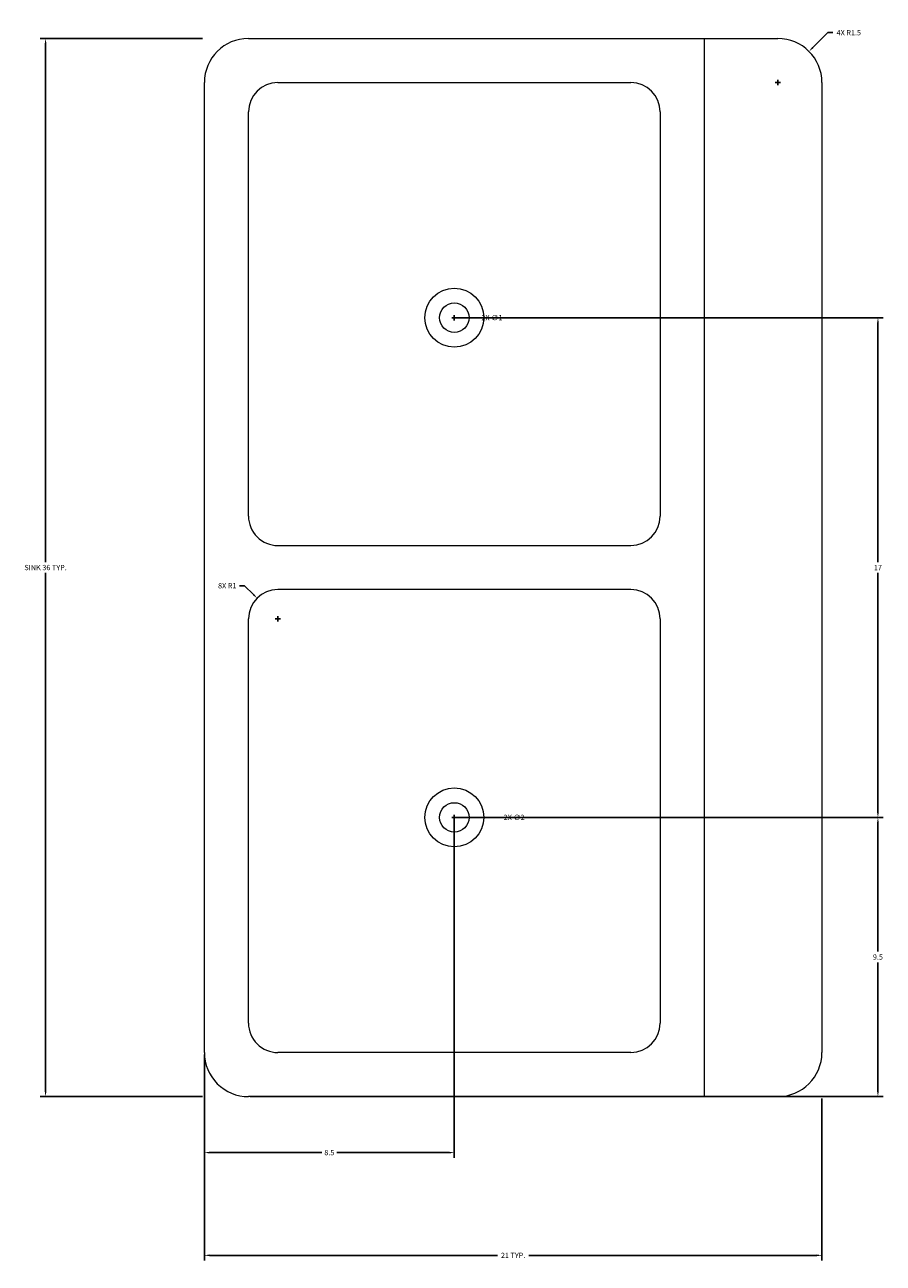
# Model space of a CAD drawing. Units: inches. Extents: x -494 to 1275, y 12 to 1194.
# Tile 8 of 8: x 1246 to 1275, y 824 to 866. Entities that reach past the tile are written whole.
import ezdxf

# ---------------------------------------------------------------- set-up
doc = ezdxf.new("R2010")
doc.units = ezdxf.units.IN
doc.header["$MEASUREMENT"] = 0
doc.layers.add('A-ANNO-DIMS', color=2, linetype='Continuous', lineweight=18)
doc.layers.add('A-FLOR-FIXT', color=8, linetype='Continuous', lineweight=18)
doc.styles.get("Standard").update_dxf_attribs({"font": 'arial.ttf'})
doc.dimstyles.get("Standard").update_dxf_attribs({"dimtxt": 0.18, "dimasz": 0.18, "dimexe": 0.18, "dimexo": 0.0625, "dimgap": 0.09, "dimtad": 0, "dimtih": 1, "dimtoh": 1, "dimdec": 4, "dimzin": 0, "dimdsep": 46, "dimlunit": 4, "dimtxsty": 'Standard', "dimcen": 0.09, "dimadec": 0, "dimazin": 0, "dimtfac": 1, "dimtdec": 4, "dimtofl": 0, "dimtmove": 0, "dimatfit": 3, "dimfxl": 1, "dimtolj": 1, "dimtzin": 0, "dimarcsym": 0})

# ---------------------------------------------------------------- blocks, each defined once
blk = doc.blocks.new('Sink-double - 36 in top')
for p, q in [((-18, -4), (18, -4)), ((-0.75, -18.5), (-0.75, -6.5)), ((0.75, -6.5), (0.75, -18.5))]:
    blk.add_line(p, q)
for points in [[(-16.5, 0), (16.5, 0)], [(-18, -19.5), (-18, -1.5)], [(18, -1.5), (18, -19.5)], [(-15.5, -5.5), (-1.75, -5.5)], [(1.75, -5.5), (15.5, -5.5)], [(-16.5, -18.5), (-16.5, -6.5)], [(16.5, -6.5), (16.5, -18.5)], [(-1.75, -19.5), (-15.5, -19.5)], [(15.5, -19.5), (1.75, -19.5)], [(16.5, -21), (-16.5, -21)]]:
    blk.add_lwpolyline(points)
for centre, radius in [((-8.5, -12.5), 1), ((8.5, -12.5), 1), ((-8.5, -12.5), 0.5), ((8.5, -12.5), 0.5)]:
    blk.add_circle(centre, radius)
for centre, radius, start, end in [((-16.5, -1.5), 1.5, 90, 180), ((16.5, -1.5), 1.5, 0, 90), ((-15.5, -6.5), 1, 90, 180), ((-1.75, -6.5), 1, 0, 90), ((1.75, -6.5), 1, 90, 180), ((15.5, -6.5), 1, 0, 90), ((-15.5, -18.5), 1, 180, 270), ((-1.75, -18.5), 1, 270, 0), ((1.75, -18.5), 1, 180, 270), ((15.5, -18.5), 1, 270, 0), ((-16.5, -19.5), 1.5, 180, 270), ((16.5, -19.5), 1.5, 270, 0)]:
    blk.add_arc(centre, radius, start, end)
blk = doc.blocks.new('*D24')
at = {"layer": 'A-ANNO-DIMS', "color": 0, "lineweight": -2, "transparency": 16777216}
for p, q in [((1252.041, 865.351), (1246.523, 865.351)), ((1246.703, 865.171), (1246.703, 847.534)), ((1246.703, 829.531), (1246.703, 847.168)), ((1252.041, 829.351), (1246.523, 829.351))]:
    blk.add_line(p, q, dxfattribs=at)
at = {"layer": 'A-ANNO-DIMS', "color": 0, "transparency": 16777216}
for points in [[(1246.673, 865.171), (1246.733, 865.171), (1246.703, 865.351)], [(1246.673, 829.531), (1246.733, 829.531), (1246.703, 829.351)]]:
    blk.add_solid(points, dxfattribs=at)
at = {"layer": 'Defpoints', "color": 0, "transparency": 16777216}
for p in [(1252.103, 865.351), (1246.703, 829.351), (1252.103, 829.351)]:
    blk.add_point(p, dxfattribs=at)
at = {"layer": 'A-ANNO-DIMS', "color": 0, "transparency": 16777216, "insert": (1246.703, 847.351), "char_height": 0.18, "attachment_point": 5}
blk.add_mtext('\\A1;SINK 36 TYP.', dxfattribs=at)
blk = doc.blocks.new('*D25')
at = {"layer": 'A-ANNO-DIMS', "color": 0, "lineweight": -2, "transparency": 16777216}
for p, q in [((1252.103, 829.289), (1252.103, 823.771)), ((1273.103, 829.289), (1273.103, 823.771)), ((1252.283, 823.951), (1262.074, 823.951)), ((1272.923, 823.951), (1263.133, 823.951))]:
    blk.add_line(p, q, dxfattribs=at)
at = {"layer": 'A-ANNO-DIMS', "color": 0, "transparency": 16777216}
for points in [[(1252.283, 823.981), (1252.283, 823.921), (1252.103, 823.951)], [(1272.923, 823.981), (1272.923, 823.921), (1273.103, 823.951)]]:
    blk.add_solid(points, dxfattribs=at)
at = {"layer": 'Defpoints', "color": 0, "transparency": 16777216}
for p in [(1252.103, 829.351), (1273.103, 829.351), (1273.103, 823.951)]:
    blk.add_point(p, dxfattribs=at)
at = {"layer": 'A-ANNO-DIMS', "color": 0, "transparency": 16777216, "insert": (1262.603, 823.951), "char_height": 0.18, "attachment_point": 5}
blk.add_mtext('\\A1;21 TYP.', dxfattribs=at)
blk = doc.blocks.new('*D75')
at = {"layer": 'A-ANNO-DIMS', "color": 0, "lineweight": -2, "transparency": 16777216}
for p, q in [((1260.666, 855.851), (1275.188, 855.851)), ((1275.008, 855.671), (1275.008, 847.531)), ((1275.008, 839.031), (1275.008, 847.171)), ((1260.666, 838.851), (1275.188, 838.851))]:
    blk.add_line(p, q, dxfattribs=at)
at = {"layer": 'A-ANNO-DIMS', "color": 0, "transparency": 16777216}
for points in [[(1274.978, 855.671), (1275.038, 855.671), (1275.008, 855.851)], [(1274.978, 839.031), (1275.038, 839.031), (1275.008, 838.851)]]:
    blk.add_solid(points, dxfattribs=at)
at = {"layer": 'Defpoints', "color": 0, "transparency": 16777216}
for p in [(1260.603, 855.851), (1275.008, 855.851), (1260.603, 838.851)]:
    blk.add_point(p, dxfattribs=at)
at = {"layer": 'A-ANNO-DIMS', "color": 0, "transparency": 16777216, "insert": (1275.008, 847.351), "char_height": 0.18, "attachment_point": 5}
blk.add_mtext('\\A1;17', dxfattribs=at)
blk = doc.blocks.new('*D93')
at = {"layer": 'A-ANNO-DIMS', "color": 0, "lineweight": -2, "transparency": 16777216}
for p, q in [((1260.603, 838.789), (1260.603, 827.266)), ((1252.103, 830.789), (1252.103, 827.266)), ((1252.283, 827.446), (1256.099, 827.446)), ((1260.423, 827.446), (1256.608, 827.446))]:
    blk.add_line(p, q, dxfattribs=at)
at = {"layer": 'A-ANNO-DIMS', "color": 0, "transparency": 16777216}
for points in [[(1252.283, 827.476), (1252.283, 827.416), (1252.103, 827.446)], [(1260.423, 827.476), (1260.423, 827.416), (1260.603, 827.446)]]:
    blk.add_solid(points, dxfattribs=at)
at = {"layer": 'Defpoints', "color": 0, "transparency": 16777216}
for p in [(1260.603, 838.851), (1252.103, 830.851), (1252.103, 827.446)]:
    blk.add_point(p, dxfattribs=at)
at = {"layer": 'A-ANNO-DIMS', "color": 0, "transparency": 16777216, "insert": (1256.353, 827.446), "char_height": 0.18, "attachment_point": 5}
blk.add_mtext('\\A1;8.5', dxfattribs=at)
blk = doc.blocks.new('*D94')
at = {"layer": 'A-ANNO-DIMS', "color": 0, "lineweight": -2, "transparency": 16777216}
for p, q in [((1260.666, 838.851), (1275.188, 838.851)), ((1275.008, 838.671), (1275.008, 834.283)), ((1275.008, 829.531), (1275.008, 833.919)), ((1253.666, 829.351), (1275.188, 829.351))]:
    blk.add_line(p, q, dxfattribs=at)
at = {"layer": 'A-ANNO-DIMS', "color": 0, "transparency": 16777216}
for points in [[(1274.978, 838.671), (1275.038, 838.671), (1275.008, 838.851)], [(1274.978, 829.531), (1275.038, 829.531), (1275.008, 829.351)]]:
    blk.add_solid(points, dxfattribs=at)
at = {"layer": 'Defpoints', "color": 0, "transparency": 16777216}
for p in [(1260.603, 838.851), (1253.603, 829.351), (1275.008, 829.351)]:
    blk.add_point(p, dxfattribs=at)
at = {"layer": 'A-ANNO-DIMS', "color": 0, "transparency": 16777216, "insert": (1275.008, 834.101), "char_height": 0.18, "attachment_point": 5}
blk.add_mtext('\\A1;9.5', dxfattribs=at)
blk = doc.blocks.new('*D105')
at = {"layer": 'A-ANNO-DIMS', "color": 0, "lineweight": -2, "transparency": 16777216}
for p, q in [((1260.603, 838.761), (1260.603, 838.941)), ((1260.513, 838.851), (1260.693, 838.851)), ((1262.203, 838.851), (1261.783, 838.851))]:
    blk.add_line(p, q, dxfattribs=at)
at = {"layer": 'A-ANNO-DIMS', "color": 0, "transparency": 16777216}
blk.add_solid([(1261.783, 838.881), (1261.783, 838.821), (1261.603, 838.851)], dxfattribs=at)
at = {"layer": 'Defpoints', "color": 0, "transparency": 16777216}
for p in [(1259.603, 838.851), (1261.603, 838.851)]:
    blk.add_point(p, dxfattribs=at)
at = {"layer": 'A-ANNO-DIMS', "color": 0, "transparency": 16777216, "insert": (1262.639, 838.851), "char_height": 0.18, "attachment_point": 5}
blk.add_mtext('\\A1;2X ∅2', dxfattribs=at)
blk = doc.blocks.new('*D106')
at = {"layer": 'A-ANNO-DIMS', "color": 0, "lineweight": -2, "transparency": 16777216}
for p, q in [((1260.513, 855.851), (1260.693, 855.851)), ((1260.603, 855.761), (1260.603, 855.941)), ((1261.463, 855.851), (1261.283, 855.851))]:
    blk.add_line(p, q, dxfattribs=at)
at = {"layer": 'A-ANNO-DIMS', "color": 0, "transparency": 16777216}
blk.add_solid([(1261.283, 855.881), (1261.283, 855.821), (1261.103, 855.851)], dxfattribs=at)
at = {"layer": 'Defpoints', "color": 0, "transparency": 16777216}
for p in [(1260.103, 855.851), (1261.103, 855.851)]:
    blk.add_point(p, dxfattribs=at)
at = {"layer": 'A-ANNO-DIMS', "color": 0, "transparency": 16777216, "insert": (1261.883, 855.851), "char_height": 0.18, "attachment_point": 5}
blk.add_mtext('\\A1;2X ∅1', dxfattribs=at)
blk = doc.blocks.new('*D107')
at = {"layer": 'A-ANNO-DIMS', "color": 0, "lineweight": -2, "transparency": 16777216}
for p, q in [((1273.3, 865.548), (1272.791, 865.039)), ((1273.48, 865.548), (1273.3, 865.548)), ((1271.513, 863.851), (1271.693, 863.851)), ((1271.603, 863.761), (1271.603, 863.941))]:
    blk.add_line(p, q, dxfattribs=at)
at = {"layer": 'A-ANNO-DIMS', "color": 0, "transparency": 16777216}
blk.add_solid([(1272.77, 865.06), (1272.812, 865.018), (1272.664, 864.912)], dxfattribs=at)
at = {"layer": 'Defpoints', "color": 0, "transparency": 16777216}
for p in [(1272.664, 864.912), (1271.603, 863.851)]:
    blk.add_point(p, dxfattribs=at)
at = {"layer": 'A-ANNO-DIMS', "color": 0, "transparency": 16777216, "insert": (1274.018, 865.548), "char_height": 0.18, "attachment_point": 5}
blk.add_mtext('\\A1;4X R1.5', dxfattribs=at)
blk = doc.blocks.new('*D108')
at = {"layer": 'A-ANNO-DIMS', "color": 0, "lineweight": -2, "transparency": 16777216}
for p, q in [((1253.292, 846.732), (1253.472, 846.732)), ((1253.472, 846.732), (1253.769, 846.435)), ((1254.603, 845.511), (1254.603, 845.691)), ((1254.513, 845.601), (1254.693, 845.601))]:
    blk.add_line(p, q, dxfattribs=at)
at = {"layer": 'A-ANNO-DIMS', "color": 0, "transparency": 16777216}
blk.add_solid([(1253.79, 846.457), (1253.747, 846.414), (1253.896, 846.308)], dxfattribs=at)
at = {"layer": 'Defpoints', "color": 0, "transparency": 16777216}
for p in [(1253.896, 846.308), (1254.603, 845.601)]:
    blk.add_point(p, dxfattribs=at)
at = {"layer": 'A-ANNO-DIMS', "color": 0, "transparency": 16777216, "insert": (1252.88, 846.732), "char_height": 0.18, "attachment_point": 5}
blk.add_mtext('\\A1;8X R1', dxfattribs=at)

msp = doc.modelspace()

# ---------------------------------------------------------------- block references
at = {"layer": 'A-FLOR-FIXT', "rotation": 270}
msp.add_blockref('Sink-double - 36 in top', (1273.1032, 847.3511), dxfattribs=at)

# ---------------------------------------------------------------- dimensions: what is measured, and where the dimension line sits
at = {"layer": 'A-ANNO-DIMS'}
for center, mpoint, text, override, picture, middle in [((1271.6032, 863.8511), (1272.6638, 864.9118), '4X <>', {"dimdec": 1, "dimlfac": 1, "dimrnd": 0, "dimzin": 0, "dimdsep": 46, "dimlunit": 2}, '*D107', (1274.0178, 865.5482)), ((1254.6032, 845.6011), (1253.8959, 846.3081), '8X <>', {"dimdec": 0, "dimlfac": 1, "dimrnd": 0, "dimzin": 0, "dimdsep": 46, "dimlunit": 2}, '*D108', (1252.8803, 846.7323))]:
    dim = msp.add_radius_dim(center=center, mpoint=mpoint, text=text, dimstyle='Standard', override=override, dxfattribs=at)
    dim.commit()
    dim.dimension.update_dxf_attribs({"geometry": picture, "text_midpoint": middle, "dimtype": 164})
dim = msp.add_linear_dim(base=(1246.7032, 829.3511), p1=(1252.1032, 865.3511), p2=(1252.1032, 829.3511), angle=270, text='SINK <> TYP.', dimstyle='Standard', override={"dimdec": 0, "dimlfac": 1, "dimrnd": 0, "dimzin": 0, "dimdsep": 46, "dimlunit": 2}, dxfattribs=at)
dim.commit()
dim.dimension.update_dxf_attribs({"geometry": '*D24', "text_midpoint": (1246.7032, 847.3511)})
dim = msp.add_diameter_dim_2p(p1=(1260.1032, 855.8512), p2=(1261.1032, 855.851), text='2X <>', dimstyle='Standard', override={"dimdec": 0, "dimlfac": 1, "dimrnd": 0, "dimzin": 0, "dimdsep": 46, "dimlunit": 2}, dxfattribs=at)
dim.commit()
dim.dimension.update_dxf_attribs({"geometry": '*D106', "text_midpoint": (1261.4632, 855.8509)})
for base, p2, override, picture, middle in [((1275.0082, 855.8511), (1260.6032, 855.8511), {"dimdec": 0, "dimlfac": 1, "dimrnd": 0, "dimzin": 0, "dimdsep": 46, "dimlunit": 2}, '*D75', (1275.0082, 847.3511)), ((1275.0082, 829.3511), (1253.6032, 829.3511), {"dimdec": 1, "dimlfac": 1, "dimrnd": 0, "dimzin": 0, "dimdsep": 46, "dimlunit": 2}, '*D94', (1275.0082, 834.1011))]:
    dim = msp.add_linear_dim(base=base, p1=(1260.6032, 838.8511), p2=p2, angle=90, dimstyle='Standard', override=override, dxfattribs=at)
    dim.commit()
    dim.dimension.update_dxf_attribs({"geometry": picture, "text_midpoint": middle})
dim = msp.add_diameter_dim_2p(p1=(1259.6032, 838.8512), p2=(1261.6032, 838.851), text='2X <>', dimstyle='Standard', override={"dimdec": 0, "dimlfac": 1, "dimrnd": 0, "dimzin": 0, "dimdsep": 46, "dimlunit": 2}, dxfattribs=at)
dim.commit()
dim.dimension.update_dxf_attribs({"geometry": '*D105', "text_midpoint": (1262.2032, 838.8509), "dimtype": 163})
dim = msp.add_linear_dim(base=(1252.1032, 827.4461), p1=(1260.6032, 838.8511), p2=(1252.1032, 830.8511), dimstyle='Standard', override={"dimdec": 1, "dimlfac": 1, "dimrnd": 0, "dimzin": 0, "dimdsep": 46, "dimlunit": 2}, dxfattribs=at)
dim.commit()
dim.dimension.update_dxf_attribs({"geometry": '*D93', "text_midpoint": (1256.3532, 827.4461)})
dim = msp.add_linear_dim(base=(1273.1032, 823.9511), p1=(1252.1032, 829.3511), p2=(1273.1032, 829.3511), text='<> TYP.', dimstyle='Standard', override={"dimdec": 0, "dimlfac": 1, "dimrnd": 0, "dimzin": 0, "dimdsep": 46, "dimlunit": 2}, dxfattribs=at)
dim.commit()
dim.dimension.update_dxf_attribs({"geometry": '*D25', "text_midpoint": (1262.6032, 823.9511)})

doc.saveas('drawing.dxf')
